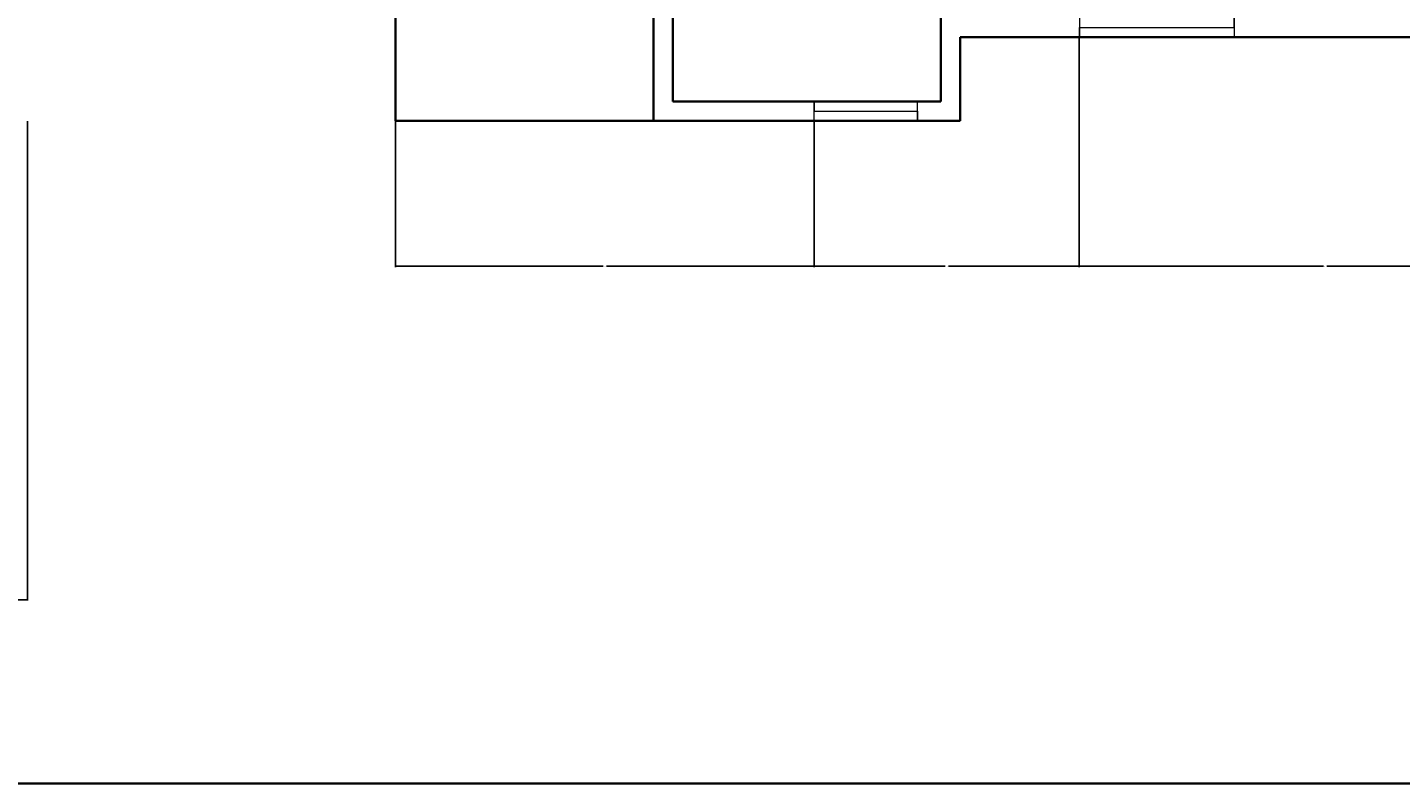
# Model space of a CAD drawing. Units: inches. Extents: x 992 to 2287, y 1476 to 2866.
# Tile 3 of 9: x 1531 to 1851, y 1476 to 1652. Entities that reach past the tile are written whole.
import ezdxf

# ---------------------------------------------------------------- set-up
doc = ezdxf.new("R2010")
doc.units = ezdxf.units.IN
for name, color, linetype, lineweight in [('A-ANNO-DIMS', 2, 'Continuous', 18), ('A-ANNO-TTLB', 7, 'Continuous', 35), ('A-GLAZ', 4, 'Continuous', 18), ('A-WALL', 7, 'Continuous', 35)]:
    doc.layers.add(name, color=color, linetype=linetype, lineweight=lineweight)
doc.styles.get("Standard").update_dxf_attribs({"font": 'arial.ttf'})
doc.dimstyles.get("Standard").update_dxf_attribs({"dimtxt": 0.18, "dimasz": 0.18, "dimexe": 0.18, "dimexo": 0.0625, "dimgap": 0.09, "dimtad": 0, "dimtih": 1, "dimtoh": 1, "dimdec": 4, "dimzin": 0, "dimdsep": 46, "dimtxsty": 'Standard', "dimcen": 0.09, "dimadec": 0, "dimazin": 0, "dimtfac": 1, "dimtdec": 4, "dimtofl": 0, "dimtmove": 0, "dimatfit": 3, "dimfxl": 1, "dimtolj": 1, "dimtzin": 0, "dimarcsym": 0})

# ---------------------------------------------------------------- blocks, each defined once
blk = doc.blocks.new('WINDOW-24IN-A')
for p, q in [((0, 24), (4.5, 24)), ((4.5, 24), (2.25, 24)), ((2.25, 24), (2.25, 0)), ((2.25, 0), (0, 0)), ((0, 0), (4.5, 0))]:
    blk.add_line(p, q)
blk = doc.blocks.new('WINDOW-36IN')
for p, q in [((0, 4.5), (0, 0)), ((36, 2.25), (36, 4.5)), ((36, 4.5), (36, 0)), ((0, 0), (0, 2.25)), ((0, 2.25), (36, 2.25))]:
    blk.add_line(p, q)
blk = doc.blocks.new('*D109')
at = {"layer": 'A-ANNO-DIMS', "color": 0, "lineweight": -2, "transparency": 16777216}
for p, q in [((1100.79, 1630.48), (1100.79, 1518.97)), ((1531.29, 1630.48), (1531.29, 1518.97)), ((1100.97, 1519.15), (1315.65, 1519.15)), ((1531.11, 1519.15), (1316.44, 1519.15))]:
    blk.add_line(p, q, dxfattribs=at)
at = {"layer": 'A-ANNO-DIMS', "color": 0, "transparency": 16777216}
for points in [[(1100.97, 1519.18), (1100.97, 1519.12), (1100.79, 1519.15)], [(1531.11, 1519.18), (1531.11, 1519.12), (1531.29, 1519.15)]]:
    blk.add_solid(points, dxfattribs=at)
at = {"layer": 'Defpoints', "color": 0, "transparency": 16777216}
for p in [(1100.79, 1630.54), (1531.29, 1630.54), (1531.29, 1519.15)]:
    blk.add_point(p, dxfattribs=at)
at = {"layer": 'A-ANNO-DIMS', "color": 0, "transparency": 16777216, "insert": (1316.04, 1519.15), "char_height": 0.18, "attachment_point": 5}
blk.add_mtext('\\A1;430.5', dxfattribs=at)
blk = doc.blocks.new('*D117')
at = {"layer": 'A-ANNO-DIMS', "color": 0, "lineweight": -2, "transparency": 16777216}
for p, q in [((1616.89, 1630.48), (1616.89, 1596.56)), ((1714.26, 1630.48), (1714.26, 1596.56)), ((1617.07, 1596.74), (1665.18, 1596.74)), ((1714.08, 1596.74), (1665.97, 1596.74))]:
    blk.add_line(p, q, dxfattribs=at)
at = {"layer": 'A-ANNO-DIMS', "color": 0, "transparency": 16777216}
for points in [[(1617.07, 1596.77), (1617.07, 1596.71), (1616.89, 1596.74)], [(1714.08, 1596.77), (1714.08, 1596.71), (1714.26, 1596.74)]]:
    blk.add_solid(points, dxfattribs=at)
at = {"layer": 'Defpoints', "color": 0, "transparency": 16777216}
for p in [(1616.89, 1630.54), (1714.26, 1630.54), (1714.26, 1596.74)]:
    blk.add_point(p, dxfattribs=at)
at = {"layer": 'A-ANNO-DIMS', "color": 0, "transparency": 16777216, "insert": (1665.57, 1596.74), "char_height": 0.18, "attachment_point": 5}
blk.add_mtext('\\A1;97.36', dxfattribs=at)
blk = doc.blocks.new('*D118')
at = {"layer": 'A-ANNO-DIMS', "color": 0, "lineweight": -2, "transparency": 16777216}
for p, q in [((1775.9, 1649.98), (1775.9, 1596.56)), ((1714.26, 1630.48), (1714.26, 1596.56)), ((1714.44, 1596.74), (1744.68, 1596.74)), ((1775.72, 1596.74), (1745.47, 1596.74))]:
    blk.add_line(p, q, dxfattribs=at)
at = {"layer": 'A-ANNO-DIMS', "color": 0, "transparency": 16777216}
for points in [[(1714.44, 1596.77), (1714.44, 1596.71), (1714.26, 1596.74)], [(1775.72, 1596.77), (1775.72, 1596.71), (1775.9, 1596.74)]]:
    blk.add_solid(points, dxfattribs=at)
at = {"layer": 'Defpoints', "color": 0, "transparency": 16777216}
for p in [(1775.9, 1650.04), (1714.26, 1630.54), (1775.9, 1596.74)]:
    blk.add_point(p, dxfattribs=at)
at = {"layer": 'A-ANNO-DIMS', "color": 0, "transparency": 16777216, "insert": (1745.08, 1596.74), "char_height": 0.18, "attachment_point": 5}
blk.add_mtext('\\A1;61.65', dxfattribs=at)
blk = doc.blocks.new('*D119')
at = {"layer": 'A-ANNO-DIMS', "color": 0, "lineweight": -2, "transparency": 16777216}
for p, q in [((1775.9, 1649.98), (1775.9, 1596.56)), ((1890.29, 1649.98), (1890.29, 1596.56)), ((1776.08, 1596.74), (1832.71, 1596.74)), ((1890.11, 1596.74), (1833.48, 1596.74))]:
    blk.add_line(p, q, dxfattribs=at)
at = {"layer": 'A-ANNO-DIMS', "color": 0, "transparency": 16777216}
for points in [[(1776.08, 1596.77), (1776.08, 1596.71), (1775.9, 1596.74)], [(1890.11, 1596.77), (1890.11, 1596.71), (1890.29, 1596.74)]]:
    blk.add_solid(points, dxfattribs=at)
at = {"layer": 'Defpoints', "color": 0, "transparency": 16777216}
for p in [(1775.9, 1650.04), (1890.29, 1650.04), (1890.29, 1596.74)]:
    blk.add_point(p, dxfattribs=at)
at = {"layer": 'A-ANNO-DIMS', "color": 0, "transparency": 16777216, "insert": (1833.1, 1596.74), "char_height": 0.18, "attachment_point": 5}
blk.add_mtext('\\A1;114.4', dxfattribs=at)

msp = doc.modelspace()

# ---------------------------------------------------------------- linework, layer by layer
at = {"layer": 'A-ANNO-TTLB'}
msp.add_lwpolyline([(992.3484, 2866.1952), (2287.217, 2866.1952), (2287.217, 1476.4066), (992.3484, 1476.4066)], close=True, dxfattribs=at)
at = {"layer": 'A-WALL'}
for p, q in [((1616.8946, 1677.0428), (1616.8946, 1630.5428)), ((1676.8946, 1677.0428), (1676.8946, 1630.5428)), ((1681.3946, 1635.0428), (1681.3946, 1677.0428)), ((1743.6835, 1677.0428), (1743.6835, 1635.0428)), ((1748.1835, 1650.0428), (1948.3946, 1650.0428)), ((1748.1835, 1650.0428), (1748.1835, 1630.5428)), ((1681.3946, 1635.0428), (1743.6835, 1635.0428)), ((1616.8946, 1630.5428), (1748.1835, 1630.5428))]:
    msp.add_line(p, q, dxfattribs=at)

# ---------------------------------------------------------------- block references
at = {"layer": 'A-GLAZ'}
msp.add_blockref('WINDOW-36IN', (1775.904, 1650.043), dxfattribs=at)
at = {"layer": 'A-GLAZ', "rotation": 90}
msp.add_blockref('WINDOW-24IN-A', (1738.2548, 1630.5432), dxfattribs=at)

# ---------------------------------------------------------------- dimensions: what is measured, and where the dimension line sits
at = {"layer": 'A-ANNO-DIMS'}
for base, p1, p2, override, picture, middle in [((1775.9038, 1596.7428), (1714.2551, 1630.5428), (1775.9038, 1650.0428), {"dimdec": 2, "dimlfac": 1, "dimrnd": 0, "dimzin": 0, "dimdsep": 46, "dimlunit": 2}, '*D118', (1745.0795, 1596.7428)), ((1890.2943, 1596.7428), (1775.9038, 1650.0428), (1890.2943, 1650.0428), {"dimdec": 1, "dimlfac": 1, "dimrnd": 0, "dimzin": 0, "dimdsep": 46, "dimlunit": 2}, '*D119', (1833.0991, 1596.7428)), ((1531.2936, 1519.1506), (1100.7936, 1630.5428), (1531.2936, 1630.5428), {"dimdec": 1, "dimlfac": 1, "dimrnd": 0, "dimzin": 0, "dimdsep": 46, "dimlunit": 2}, '*D109', (1316.0436, 1519.1506)), ((1714.2551, 1596.7428), (1616.8946, 1630.5428), (1714.2551, 1630.5428), {"dimdec": 2, "dimlfac": 1, "dimrnd": 0, "dimzin": 0, "dimdsep": 46, "dimlunit": 2}, '*D117', (1665.5749, 1596.7428))]:
    dim = msp.add_linear_dim(base=base, p1=p1, p2=p2, dimstyle='Standard', override=override, dxfattribs=at)
    dim.commit()
    dim.dimension.update_dxf_attribs({"geometry": picture, "text_midpoint": middle})

doc.saveas('drawing.dxf')
